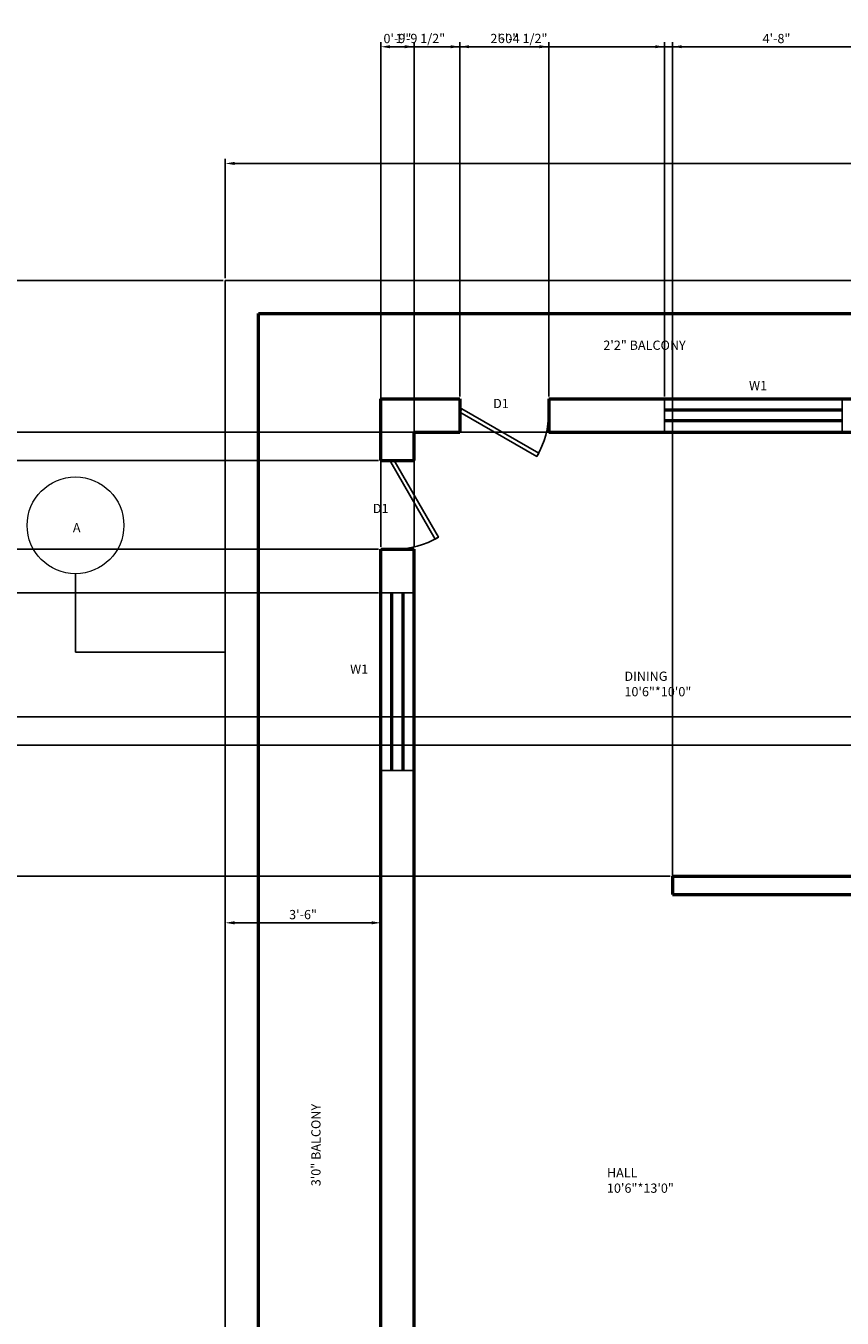
# Model space of a CAD drawing. Units: inches. Extents: x 2020 to 7901, y 1581 to 3943.
# Tile 4 of 17: x 2305 to 2526, y 1966 to 2315. Entities that reach past the tile are written whole.
import ezdxf

# ---------------------------------------------------------------- set-up
doc = ezdxf.new("R2010")
doc.units = ezdxf.units.IN
for name, color, linetype, lineweight in [('A-ANNO-DIMS', 2, 'Continuous', 18), ('A-ANNO-SYMB', 1, 'Continuous', 18), ('A-ANNO-TEXT', 7, 'Continuous', 18), ('A-AREA-IDEN', 3, 'Continuous', 18), ('A-DOOR', 4, 'Continuous', 25), ('A-GLAZ', 4, 'Continuous', 25), ('A-WALL', 7, 'Continuous', 50), ('C-PROP', 6, 'Continuous', 25)]:
    doc.layers.add(name, color=color, linetype=linetype, lineweight=lineweight)
doc.styles.get("Standard").update_dxf_attribs({"font": 'arial.ttf'})
doc.dimstyles.new('ISO-25', dxfattribs={"dimtxt": 2.5, "dimasz": 2.5, "dimexe": 1.25, "dimexo": 0.625, "dimtad": 1, "dimdec": 1, "dimlunit": 3, "dimtxsty": 'Standard', "dimcen": 2.5, "dimadec": 0, "dimazin": 0, "dimtfac": 1, "dimtdec": 1, "dimtmove": 0, "dimatfit": 3, "dimfxl": 1, "dimarcsym": 0})

# ---------------------------------------------------------------- blocks, each defined once
blk = doc.blocks.new('*U2')
for p, q in [((0, 0), (0, -6)), ((40, 0), (40, -6))]:
    blk.add_line(p, q)
blk.add_lwpolyline([(0, 0), (34.64, 20), (35.52, 18.48), (0.87, -1.52)], close=True)
blk.add_arc((0, 0), 40, 0, 30)
blk = doc.blocks.new('*D4')
at = {"layer": 'A-ANNO-DIMS', "color": 0, "lineweight": -2, "transparency": 16777216}
for p, q in [((2358.34, 2246.34), (2285.83, 2246.34)), ((2287.08, 2243.84), (2287.08, 1768.84)), ((2358.34, 1766.34), (2285.83, 1766.34))]:
    blk.add_line(p, q, dxfattribs=at)
at = {"layer": 'A-ANNO-DIMS', "color": 0, "transparency": 16777216}
for points in [[(2286.66, 2243.84), (2287.49, 2243.84), (2287.08, 2246.34)], [(2286.66, 1768.84), (2287.49, 1768.84), (2287.08, 1766.34)]]:
    blk.add_solid(points, dxfattribs=at)
at = {"layer": 'DEFPOINTS', "color": 0, "transparency": 16777216}
for p in [(2358.96, 2246.34), (2287.08, 1766.34), (2358.96, 1766.34)]:
    blk.add_point(p, dxfattribs=at)
at = {"layer": 'A-ANNO-DIMS', "color": 0, "transparency": 16777216, "insert": (2285.18, 2006.34), "char_height": 2.5, "attachment_point": 5, "rotation": 90}
blk.add_mtext("40'", dxfattribs=at)
blk = doc.blocks.new('*D5')
at = {"layer": 'A-ANNO-DIMS', "color": 0, "lineweight": -2, "transparency": 16777216}
for p, q in [((2358.96, 2064.2), (2358.96, 2073.96)), ((2361.46, 2072.71), (2398.46, 2072.71)), ((2400.96, 2064.2), (2400.96, 2073.96))]:
    blk.add_line(p, q, dxfattribs=at)
at = {"layer": 'A-ANNO-DIMS', "color": 0, "transparency": 16777216}
for points in [[(2361.46, 2073.13), (2361.46, 2072.29), (2358.96, 2072.71)], [(2398.46, 2073.13), (2398.46, 2072.29), (2400.96, 2072.71)]]:
    blk.add_solid(points, dxfattribs=at)
at = {"layer": 'DEFPOINTS', "color": 0, "transparency": 16777216}
for p in [(2400.96, 2072.71), (2358.96, 2063.58), (2400.96, 2063.58)]:
    blk.add_point(p, dxfattribs=at)
at = {"layer": 'A-ANNO-DIMS', "color": 0, "transparency": 16777216, "insert": (2379.96, 2074.61), "char_height": 2.5, "attachment_point": 5}
blk.add_mtext('3\'-6"', dxfattribs=at)
blk = doc.blocks.new('*D8')
at = {"layer": 'A-ANNO-DIMS', "color": 0, "lineweight": -2, "transparency": 16777216}
for p, q in [((2358.96, 2246.96), (2358.96, 2279.19)), ((2361.46, 2277.94), (2716.46, 2277.94)), ((2718.96, 2246.96), (2718.96, 2279.19))]:
    blk.add_line(p, q, dxfattribs=at)
at = {"layer": 'A-ANNO-DIMS', "color": 0, "transparency": 16777216}
for points in [[(2361.46, 2278.35), (2361.46, 2277.52), (2358.96, 2277.94)], [(2716.46, 2278.35), (2716.46, 2277.52), (2718.96, 2277.94)]]:
    blk.add_solid(points, dxfattribs=at)
at = {"layer": 'DEFPOINTS', "color": 0, "transparency": 16777216}
for p in [(2718.96, 2277.94), (2358.96, 2246.34), (2718.96, 2246.34)]:
    blk.add_point(p, dxfattribs=at)
at = {"layer": 'A-ANNO-DIMS', "color": 0, "transparency": 16777216, "insert": (2538.96, 2279.84), "char_height": 2.5, "attachment_point": 5}
blk.add_mtext("30'", dxfattribs=at)
blk = doc.blocks.new('WIN-1200')
for p, q in [((0, 9), (48, 9)), ((0, 0), (0, 9)), ((48, 9), (48, 0)), ((48, 0), (0, 0))]:
    blk.add_line(p, q)
blk = doc.blocks.new('*D31')
at = {"layer": 'A-ANNO-DIMS', "color": 0, "lineweight": -2, "transparency": 16777216}
for p, q in [((2400.96, 2214.96), (2400.96, 2310.73)), ((2403.46, 2309.48), (2475.11, 2309.48)), ((2477.61, 2214.96), (2477.61, 2310.73))]:
    blk.add_line(p, q, dxfattribs=at)
at = {"layer": 'A-ANNO-DIMS', "color": 0, "transparency": 16777216}
for points in [[(2403.46, 2309.9), (2403.46, 2309.07), (2400.96, 2309.48)], [(2475.11, 2309.9), (2475.11, 2309.07), (2477.61, 2309.48)]]:
    blk.add_solid(points, dxfattribs=at)
at = {"layer": 'DEFPOINTS', "color": 0, "transparency": 16777216}
for p in [(2477.61, 2309.48), (2400.96, 2214.34), (2477.61, 2214.34)]:
    blk.add_point(p, dxfattribs=at)
at = {"layer": 'A-ANNO-DIMS', "color": 0, "transparency": 16777216, "insert": (2439.29, 2311.4), "char_height": 2.5, "attachment_point": 5}
blk.add_mtext('6\'-4 1/2"', dxfattribs=at)
blk = doc.blocks.new('*D41')
at = {"layer": 'A-ANNO-DIMS', "color": 0, "lineweight": -2, "transparency": 16777216}
for p, q in [((2400.34, 2197.7), (2272.67, 2197.7)), ((2273.92, 2195.2), (2273.92, 2176.2)), ((2400.34, 2173.7), (2272.67, 2173.7))]:
    blk.add_line(p, q, dxfattribs=at)
at = {"layer": 'A-ANNO-DIMS', "color": 0, "transparency": 16777216}
for points in [[(2273.5, 2195.2), (2274.33, 2195.2), (2273.92, 2197.7)], [(2273.5, 2176.2), (2274.33, 2176.2), (2273.92, 2173.7)]]:
    blk.add_solid(points, dxfattribs=at)
at = {"layer": 'DEFPOINTS', "color": 0, "transparency": 16777216}
for p in [(2400.96, 2197.7), (2273.92, 2173.7), (2400.96, 2173.7)]:
    blk.add_point(p, dxfattribs=at)
at = {"layer": 'A-ANNO-DIMS', "color": 0, "transparency": 16777216, "insert": (2272.01, 2185.7), "char_height": 2.5, "attachment_point": 5, "rotation": 90}
blk.add_mtext('2\'-0"', dxfattribs=at)
blk = doc.blocks.new('*D43')
at = {"layer": 'A-ANNO-DIMS', "color": 0, "lineweight": -2, "transparency": 16777216}
for p, q in [((2400.96, 2174.32), (2400.96, 2310.73)), ((2403.46, 2309.48), (2407.46, 2309.48)), ((2409.96, 2174.32), (2409.96, 2310.73))]:
    blk.add_line(p, q, dxfattribs=at)
at = {"layer": 'A-ANNO-DIMS', "color": 0, "transparency": 16777216}
for points in [[(2403.46, 2309.9), (2403.46, 2309.07), (2400.96, 2309.48)], [(2407.46, 2309.9), (2407.46, 2309.07), (2409.96, 2309.48)]]:
    blk.add_solid(points, dxfattribs=at)
at = {"layer": 'DEFPOINTS', "color": 0, "transparency": 16777216}
for p in [(2409.96, 2309.48), (2400.96, 2173.7), (2409.96, 2173.7)]:
    blk.add_point(p, dxfattribs=at)
at = {"layer": 'A-ANNO-DIMS', "color": 0, "transparency": 16777216, "insert": (2405.46, 2311.38), "char_height": 2.5, "attachment_point": 5}
blk.add_mtext('0\'-9"', dxfattribs=at)
blk = doc.blocks.new('*D95')
at = {"layer": 'A-ANNO-DIMS', "color": 0, "lineweight": -2, "transparency": 16777216}
for p, q in [((2400.96, 2214.96), (2400.96, 2310.73)), ((2403.46, 2309.48), (2695.46, 2309.48)), ((2697.96, 2214.96), (2697.96, 2310.73))]:
    blk.add_line(p, q, dxfattribs=at)
at = {"layer": 'A-ANNO-DIMS', "color": 0, "transparency": 16777216}
for points in [[(2403.46, 2309.9), (2403.46, 2309.07), (2400.96, 2309.48)], [(2695.46, 2309.9), (2695.46, 2309.07), (2697.96, 2309.48)]]:
    blk.add_solid(points, dxfattribs=at)
at = {"layer": 'DEFPOINTS', "color": 0, "transparency": 16777216}
for p in [(2697.96, 2309.48), (2400.96, 2214.34), (2697.96, 2214.34)]:
    blk.add_point(p, dxfattribs=at)
at = {"layer": 'A-ANNO-DIMS', "color": 0, "transparency": 16777216, "insert": (2549.46, 2311.38), "char_height": 2.5, "attachment_point": 5}
blk.add_mtext('24\'-9"', dxfattribs=at)
blk = doc.blocks.new('*D97')
at = {"layer": 'A-ANNO-DIMS', "color": 0, "lineweight": -2, "transparency": 16777216}
for p, q in [((2400.96, 2214.96), (2400.96, 2310.73)), ((2403.46, 2309.48), (2419.84, 2309.48)), ((2422.34, 2214.96), (2422.34, 2310.73))]:
    blk.add_line(p, q, dxfattribs=at)
at = {"layer": 'A-ANNO-DIMS', "color": 0, "transparency": 16777216}
for points in [[(2403.46, 2309.9), (2403.46, 2309.07), (2400.96, 2309.48)], [(2419.84, 2309.9), (2419.84, 2309.07), (2422.34, 2309.48)]]:
    blk.add_solid(points, dxfattribs=at)
at = {"layer": 'DEFPOINTS', "color": 0, "transparency": 16777216}
for p in [(2422.34, 2309.48), (2400.96, 2214.34), (2422.34, 2214.34)]:
    blk.add_point(p, dxfattribs=at)
at = {"layer": 'A-ANNO-DIMS', "color": 0, "transparency": 16777216, "insert": (2411.65, 2311.4), "char_height": 2.5, "attachment_point": 5}
blk.add_mtext('1\'-9 1/2"', dxfattribs=at)
blk = doc.blocks.new('*D98')
at = {"layer": 'A-ANNO-DIMS', "color": 0, "lineweight": -2, "transparency": 16777216}
for p, q in [((2422.34, 2214.96), (2422.34, 2310.73)), ((2424.84, 2309.48), (2443.84, 2309.48)), ((2446.34, 2214.96), (2446.34, 2310.73))]:
    blk.add_line(p, q, dxfattribs=at)
at = {"layer": 'A-ANNO-DIMS', "color": 0, "transparency": 16777216}
for points in [[(2424.84, 2309.9), (2424.84, 2309.07), (2422.34, 2309.48)], [(2443.84, 2309.9), (2443.84, 2309.07), (2446.34, 2309.48)]]:
    blk.add_solid(points, dxfattribs=at)
at = {"layer": 'DEFPOINTS', "color": 0, "transparency": 16777216}
for p in [(2446.34, 2309.48), (2422.34, 2214.34), (2446.34, 2214.34)]:
    blk.add_point(p, dxfattribs=at)
at = {"layer": 'A-ANNO-DIMS', "color": 0, "transparency": 16777216, "insert": (2434.34, 2311.38), "char_height": 2.5, "attachment_point": 5}
blk.add_mtext('2\'-0"', dxfattribs=at)
blk = doc.blocks.new('*D106')
at = {"layer": 'A-ANNO-DIMS', "color": 0, "lineweight": -2, "transparency": 16777216}
for p, q in [((2476.99, 2205.34), (2272.67, 2205.34)), ((2273.92, 2202.84), (2273.92, 2087.84)), ((2479.18, 2085.34), (2272.67, 2085.34))]:
    blk.add_line(p, q, dxfattribs=at)
at = {"layer": 'A-ANNO-DIMS', "color": 0, "transparency": 16777216}
for points in [[(2273.5, 2202.84), (2274.33, 2202.84), (2273.92, 2205.34)], [(2273.5, 2087.84), (2274.33, 2087.84), (2273.92, 2085.34)]]:
    blk.add_solid(points, dxfattribs=at)
at = {"layer": 'DEFPOINTS', "color": 0, "transparency": 16777216}
for p in [(2477.61, 2205.34), (2273.92, 2085.34), (2479.8, 2085.34)]:
    blk.add_point(p, dxfattribs=at)
at = {"layer": 'A-ANNO-DIMS', "color": 0, "transparency": 16777216, "insert": (2272.01, 2145.34), "char_height": 2.5, "attachment_point": 5, "rotation": 90}
blk.add_mtext('10\'-0"', dxfattribs=at)
blk = doc.blocks.new('*D107')
at = {"layer": 'A-ANNO-DIMS', "color": 0, "lineweight": -2, "transparency": 16777216}
for p, q in [((2479.8, 2080.96), (2479.8, 2310.73)), ((2482.3, 2309.48), (2533.46, 2309.48)), ((2535.96, 2080.96), (2535.96, 2310.73))]:
    blk.add_line(p, q, dxfattribs=at)
at = {"layer": 'A-ANNO-DIMS', "color": 0, "transparency": 16777216}
for points in [[(2482.3, 2309.9), (2482.3, 2309.07), (2479.8, 2309.48)], [(2533.46, 2309.9), (2533.46, 2309.07), (2535.96, 2309.48)]]:
    blk.add_solid(points, dxfattribs=at)
at = {"layer": 'DEFPOINTS', "color": 0, "transparency": 16777216}
for p in [(2535.96, 2309.48), (2479.8, 2080.34), (2535.96, 2080.34)]:
    blk.add_point(p, dxfattribs=at)
at = {"layer": 'A-ANNO-DIMS', "color": 0, "transparency": 16777216, "insert": (2507.88, 2311.38), "char_height": 2.5, "attachment_point": 5}
blk.add_mtext('4\'-8"', dxfattribs=at)
blk = doc.blocks.new('*D111')
at = {"layer": 'A-ANNO-DIMS', "color": 0, "lineweight": -2, "transparency": 16777216}
for p, q in [((2540.34, 2128.34), (2272.67, 2128.34)), ((2273.92, 2125.84), (2273.92, 2123.23)), ((2540.34, 2120.73), (2272.67, 2120.73)), ((2273.92, 2120.73), (2273.92, 2104.51))]:
    blk.add_line(p, q, dxfattribs=at)
at = {"layer": 'A-ANNO-DIMS', "color": 0, "transparency": 16777216}
for points in [[(2273.5, 2125.84), (2274.33, 2125.84), (2273.92, 2128.34)], [(2273.5, 2123.23), (2274.33, 2123.23), (2273.92, 2120.73)]]:
    blk.add_solid(points, dxfattribs=at)
at = {"layer": 'DEFPOINTS', "color": 0, "transparency": 16777216}
for p in [(2540.96, 2128.34), (2273.92, 2120.73), (2540.96, 2120.73)]:
    blk.add_point(p, dxfattribs=at)
at = {"layer": 'A-ANNO-DIMS', "color": 0, "transparency": 16777216, "insert": (2272, 2111.37), "char_height": 2.5, "attachment_point": 5, "rotation": 90}
blk.add_mtext('0\'-7 1/2"', dxfattribs=at)
blk = doc.blocks.new('*D118')
at = {"layer": 'A-ANNO-DIMS', "color": 0, "lineweight": -2, "transparency": 16777216}
for p, q in [((2400.34, 2173.7), (2272.67, 2173.7)), ((2273.92, 2171.2), (2273.92, 2164.37)), ((2400.34, 2161.87), (2272.67, 2161.87))]:
    blk.add_line(p, q, dxfattribs=at)
at = {"layer": 'A-ANNO-DIMS', "color": 0, "transparency": 16777216}
for points in [[(2273.5, 2171.2), (2274.33, 2171.2), (2273.92, 2173.7)], [(2273.5, 2164.37), (2274.33, 2164.37), (2273.92, 2161.87)]]:
    blk.add_solid(points, dxfattribs=at)
at = {"layer": 'DEFPOINTS', "color": 0, "transparency": 16777216}
for p in [(2400.96, 2173.7), (2273.92, 2161.87), (2400.96, 2161.87)]:
    blk.add_point(p, dxfattribs=at)
at = {"layer": 'A-ANNO-DIMS', "color": 0, "transparency": 16777216, "insert": (2272.01, 2167.79), "char_height": 2.5, "attachment_point": 5, "rotation": 90}
blk.add_mtext('1\'-0"', dxfattribs=at)

msp = doc.modelspace()

# ---------------------------------------------------------------- linework, layer by layer
at = {"layer": 'A-ANNO-SYMB'}
msp.add_circle((2318.48, 2180.13), 13.07, dxfattribs=at)
at = {"layer": 'A-WALL'}
for p, q in [((2367.96, 2237.34), (2709.96, 2237.34)), ((2367.96, 1766.34), (2367.96, 2237.34)), ((2400.96, 2214.34), (2422.34, 2214.34)), ((2400.96, 2197.7), (2400.96, 2214.34)), ((2422.34, 2214.34), (2422.34, 2205.34)), ((2446.34, 2214.34), (2446.34, 2205.34)), ((2446.34, 2214.34), (2697.96, 2214.34)), ((2477.61, 2211.34), (2525.61, 2211.34)), ((2525.61, 2208.34), (2477.61, 2208.34)), ((2409.96, 2205.34), (2422.34, 2205.34)), ((2409.96, 2197.7), (2409.96, 2205.34)), ((2446.34, 2205.34), (2535.96, 2205.34)), ((2400.96, 2197.7), (2409.96, 2197.7)), ((2400.96, 1919.34), (2400.96, 2173.7)), ((2400.96, 2173.7), (2409.96, 2173.7)), ((2409.96, 1924.34), (2409.96, 2173.7)), ((2403.96, 2113.87), (2403.96, 2161.87)), ((2406.96, 2161.87), (2406.96, 2113.87)), ((2479.8, 2085.34), (2535.96, 2085.34)), ((2479.8, 2085.34), (2479.8, 2080.34)), ((2479.8, 2080.34), (2535.96, 2080.34))]:
    msp.add_line(p, q, dxfattribs=at)
at = {"layer": 'C-PROP'}
for p, q in [((2358.96, 2246.34), (2718.96, 2246.34)), ((2358.96, 1766.34), (2358.96, 2246.34)), ((2318.48, 2145.81), (2318.48, 2167.06)), ((2358.96, 2145.81), (2318.48, 2145.81))]:
    msp.add_line(p, q, dxfattribs=at)

# ---------------------------------------------------------------- block references
at = {"layer": 'A-DOOR', "yscale": 0.6, "zscale": 0.6}
for p, xscale, rotation in [((2422.34, 2210.74), -0.6, 180), ((2404.56, 2197.7), 0.6, 270)]:
    msp.add_blockref('*U2', p, dxfattribs=dict(at, xscale=xscale, rotation=rotation))
at = {"layer": 'A-GLAZ'}
msp.add_blockref('WIN-1200', (2477.61, 2205.34), dxfattribs=at)
at = {"layer": 'A-GLAZ', "rotation": 90.00000000000003}
msp.add_blockref('WIN-1200', (2409.97, 2113.87), dxfattribs=at)

# ---------------------------------------------------------------- texts
at = {"layer": 'A-ANNO-SYMB', "insert": (2317.77, 2180.75), "char_height": 2.5, "attachment_point": 1}
msp.add_mtext_dynamic_manual_height_columns('A', width=12.7156, gutter_width=12.5, heights=[0], dxfattribs=at)
at = {"layer": 'A-ANNO-TEXT', "char_height": 2.5, "attachment_point": 1}
for s, width, insert in [('2\'2" BALCONY', 73.3896, (2461.09, 2230.06)), ('W1', 16.526, (2500.45, 2219.16)), ('D1', 7.9594, (2431.32, 2214.31)), ('D1', 5.9868, (2398.82, 2185.94)), ('W1', 9.2868, (2392.68, 2142.52))]:
    msp.add_mtext_dynamic_manual_height_columns(s, width=width, gutter_width=12.5, heights=[0], dxfattribs=dict(at, insert=insert))
at = {"layer": 'A-ANNO-TEXT', "insert": (2382.19, 2001.51), "char_height": 2.5, "attachment_point": 1, "rotation": 90}
msp.add_mtext_dynamic_manual_height_columns('3\'0" BALCONY', width=25.1036, gutter_width=12.5, heights=[0], dxfattribs=at)
at = {"layer": 'A-AREA-IDEN', "char_height": 2.5, "attachment_point": 1}
for s, width, insert in [('DINING\\P10\'6"*10\'0"', 76.3715, (2466.79, 2140.6)), ('HALL\\P10\'6"*13\'0"', 68.253, (2462.07, 2006.41))]:
    msp.add_mtext_dynamic_manual_height_columns(s, width=width, gutter_width=12.5, heights=[0], dxfattribs=dict(at, insert=insert))

# ---------------------------------------------------------------- dimensions: what is measured, and where the dimension line sits
at = {"layer": 'A-ANNO-DIMS'}
for base, p1, p2, override, picture, middle in [((2477.6148, 2309.4828), (2400.9649, 2214.3394), (2477.6148, 2214.3394), {"dimdec": 1, "dimlfac": 1, "dimrnd": 0, "dimzin": 1, "dimdsep": 46, "dimlunit": 4, "dimfrac": 2}, '*D31', (2439.2899, 2311.4005)), ((2422.34, 2309.48), (2400.96, 2214.34), (2422.34, 2214.34), {"dimdec": 1, "dimlfac": 1, "dimrnd": 0, "dimzin": 1, "dimdsep": 46, "dimlunit": 4, "dimfrac": 2}, '*D97', (2411.65, 2311.4)), ((2409.96, 2309.48), (2400.96, 2173.7), (2409.96, 2173.7), {"dimdec": 1, "dimlfac": 1, "dimrnd": 0, "dimzin": 1, "dimdsep": 46, "dimlunit": 4, "dimfrac": 2}, '*D43', (2405.46, 2311.38)), ((2697.96, 2309.48), (2400.96, 2214.34), (2697.96, 2214.34), {"dimdec": 1, "dimlfac": 1, "dimrnd": 0, "dimzin": 1, "dimdsep": 46, "dimlunit": 4, "dimfrac": 2}, '*D95', (2549.46, 2311.38)), ((2446.34, 2309.48), (2422.34, 2214.34), (2446.34, 2214.34), {"dimdec": 1, "dimlfac": 1, "dimrnd": 0, "dimzin": 1, "dimdsep": 46, "dimlunit": 4, "dimfrac": 2}, '*D98', (2434.34, 2311.38)), ((2535.96, 2309.48), (2479.8, 2080.34), (2535.96, 2080.34), {"dimdec": 1, "dimlfac": 1, "dimrnd": 0, "dimzin": 1, "dimdsep": 46, "dimlunit": 4, "dimfrac": 2}, '*D107', (2507.88, 2311.38)), ((2718.96, 2277.94), (2358.96, 2246.34), (2718.96, 2246.34), {"dimclrd": 0, "dimclre": 0, "dimclrt": 0}, '*D8', (2538.96, 2279.84)), ((2400.96, 2072.71), (2358.96, 2063.58), (2400.96, 2063.58), {"dimclrd": 0, "dimclre": 0, "dimclrt": 0}, '*D5', (2379.96, 2074.61))]:
    dim = msp.add_linear_dim(base=base, p1=p1, p2=p2, dimstyle='ISO-25', override=override, dxfattribs=at)
    dim.commit()
    dim.dimension.update_dxf_attribs({"geometry": picture, "text_midpoint": middle})
for base, p1, p2, override, picture, middle in [((2287.08, 1766.34), (2358.96, 2246.34), (2358.96, 1766.34), {"dimclrd": 0, "dimclre": 0, "dimclrt": 0}, '*D4', (2285.18, 2006.34)), ((2273.92, 2085.34), (2477.61, 2205.34), (2479.8, 2085.34), {"dimdec": 1, "dimlfac": 1, "dimrnd": 0, "dimzin": 1, "dimdsep": 46, "dimlunit": 4, "dimfrac": 2}, '*D106', (2272.01, 2145.34)), ((2273.92, 2173.7), (2400.96, 2197.7), (2400.96, 2173.7), {"dimdec": 1, "dimlfac": 1, "dimrnd": 0, "dimzin": 1, "dimdsep": 46, "dimlunit": 4, "dimfrac": 2}, '*D41', (2272.01, 2185.7)), ((2273.92, 2161.87), (2400.96, 2173.7), (2400.96, 2161.87), {"dimdec": 1, "dimlfac": 1, "dimrnd": 0, "dimzin": 1, "dimdsep": 46, "dimlunit": 4, "dimfrac": 2}, '*D118', (2272.01, 2167.79)), ((2273.92, 2120.73), (2540.96, 2128.34), (2540.96, 2120.73), {"dimdec": 1, "dimlfac": 1, "dimrnd": 0, "dimzin": 1, "dimdsep": 46, "dimlunit": 4, "dimfrac": 2}, '*D111', (2272, 2111.37))]:
    dim = msp.add_linear_dim(base=base, p1=p1, p2=p2, angle=90, dimstyle='ISO-25', override=override, dxfattribs=at)
    dim.commit()
    dim.dimension.update_dxf_attribs({"geometry": picture, "text_midpoint": middle})

doc.saveas('drawing.dxf')
